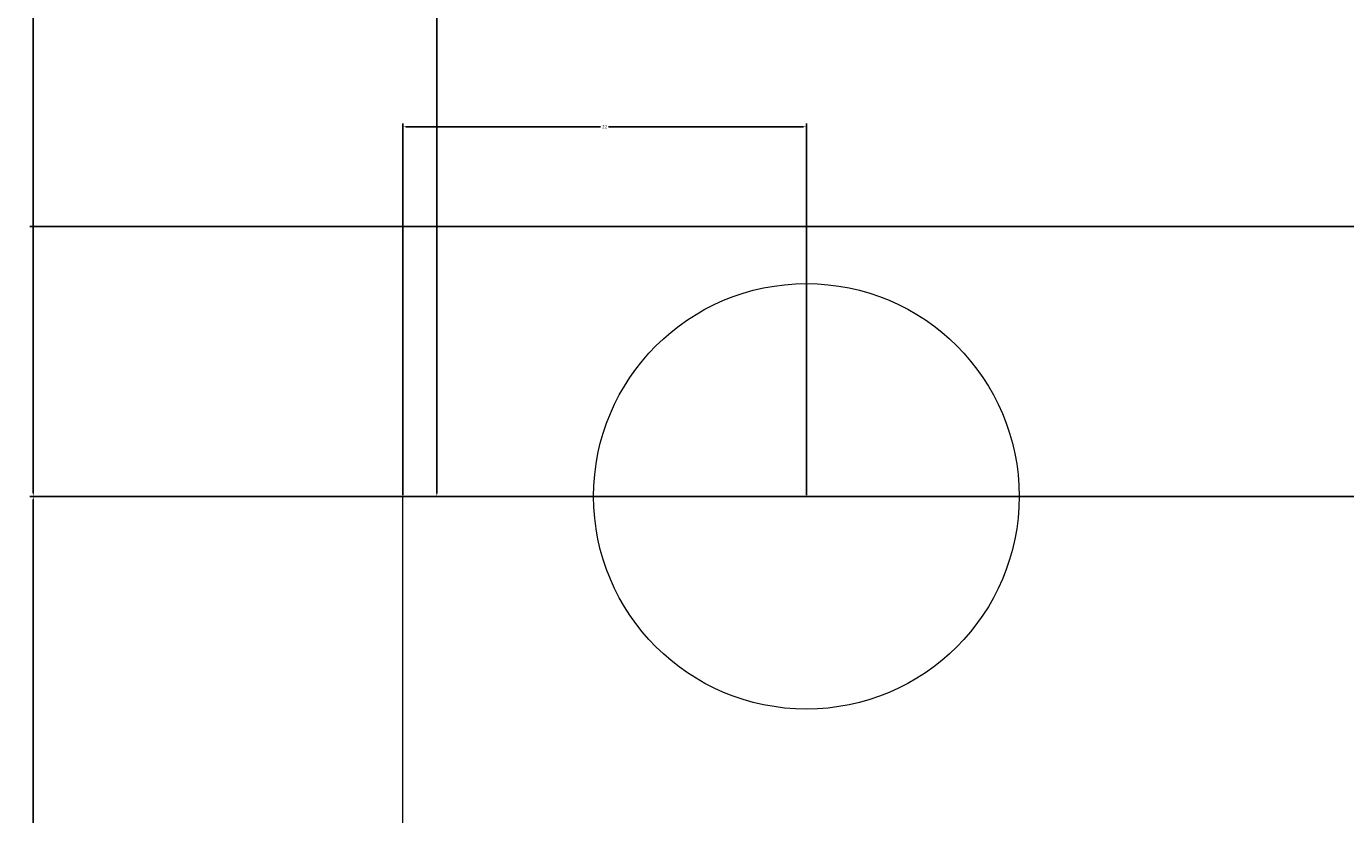
# Model space of a CAD drawing. Units: inches. Extents: x 1095 to 1408, y -20 to 240.
# Tile 2 of 8: x 1095 to 1167, y 23 to 66. Entities that reach past the tile are written whole.
import ezdxf

# ---------------------------------------------------------------- set-up
doc = ezdxf.new("R2010")
doc.units = ezdxf.units.IN
doc.header["$MEASUREMENT"] = 0
doc.layers.add('M-CONS', color=8, linetype='Continuous', lineweight=18)
doc.layers.add('M-DIMS', color=2, linetype='Continuous', lineweight=18)
doc.styles.get("Standard").update_dxf_attribs({"font": 'arial.ttf'})
doc.dimstyles.get("Standard").update_dxf_attribs({"dimtxt": 0.18, "dimasz": 0.18, "dimexe": 0.18, "dimexo": 0.0625, "dimgap": 0.09, "dimtad": 0, "dimtih": 1, "dimtoh": 1, "dimdec": 4, "dimzin": 0, "dimdsep": 46, "dimtxsty": 'Standard', "dimcen": 0.09, "dimadec": 0, "dimazin": 0, "dimtfac": 1, "dimtdec": 4, "dimtofl": 0, "dimtmove": 0, "dimatfit": 3, "dimfxl": 1, "dimtolj": 1, "dimtzin": 0, "dimarcsym": 0})

# ---------------------------------------------------------------- blocks, each defined once
blk = doc.blocks.new('*D3')
at = {"layer": 'Defpoints', "color": 0, "transparency": 16777216}
for p in [(1137.184, 60.15), (1115.184, 40), (1137.184, 40)]:
    blk.add_point(p, dxfattribs=at)
at = {"layer": 'M-DIMS', "color": 0, "lineweight": -2, "transparency": 16777216}
for p, q in [((1115.184, 40.062), (1115.184, 60.33)), ((1115.364, 60.15), (1125.964, 60.15)), ((1137.004, 60.15), (1126.403, 60.15)), ((1137.184, 40.062), (1137.184, 60.33))]:
    blk.add_line(p, q, dxfattribs=at)
at = {"layer": 'M-DIMS', "color": 0, "transparency": 16777216}
for points in [[(1115.364, 60.18), (1115.364, 60.12), (1115.184, 60.15)], [(1137.004, 60.18), (1137.004, 60.12), (1137.184, 60.15)]]:
    blk.add_solid(points, dxfattribs=at)
at = {"layer": 'M-DIMS', "color": 0, "transparency": 16777216, "insert": (1126.184, 60.15), "char_height": 0.18, "attachment_point": 5}
blk.add_mtext('\\A1;22', dxfattribs=at)
blk = doc.blocks.new('*D4')
at = {"layer": 'Defpoints', "color": 0, "transparency": 16777216}
for p in [(1095.034, 40), (1115.184, 40), (1115.184, 0)]:
    blk.add_point(p, dxfattribs=at)
at = {"layer": 'M-DIMS', "color": 0, "lineweight": -2, "transparency": 16777216}
for p, q in [((1115.121, 40), (1094.854, 40)), ((1095.034, 39.82), (1095.034, 20.182)), ((1095.034, 0.18), (1095.034, 19.818)), ((1115.121, 0), (1094.854, 0))]:
    blk.add_line(p, q, dxfattribs=at)
at = {"layer": 'M-DIMS', "color": 0, "transparency": 16777216}
for points in [[(1095.004, 39.82), (1095.064, 39.82), (1095.034, 40)], [(1095.004, 0.18), (1095.064, 0.18), (1095.034, 0)]]:
    blk.add_solid(points, dxfattribs=at)
at = {"layer": 'M-DIMS', "color": 0, "transparency": 16777216, "insert": (1095.034, 20), "char_height": 0.18, "attachment_point": 5}
blk.add_mtext('\\A1;40', dxfattribs=at)
blk = doc.blocks.new('*D6')
at = {"layer": 'Defpoints', "color": 0, "transparency": 16777216}
for p in [(1117.034, 208), (1137.184, 208), (1137.184, 40)]:
    blk.add_point(p, dxfattribs=at)
at = {"layer": 'M-DIMS', "color": 0, "lineweight": -2, "transparency": 16777216}
for p, q in [((1137.121, 208), (1116.854, 208)), ((1117.034, 207.82), (1117.034, 124.182)), ((1117.034, 40.18), (1117.034, 123.818)), ((1137.121, 40), (1116.854, 40))]:
    blk.add_line(p, q, dxfattribs=at)
at = {"layer": 'M-DIMS', "color": 0, "transparency": 16777216}
for points in [[(1117.004, 207.82), (1117.064, 207.82), (1117.034, 208)], [(1117.004, 40.18), (1117.064, 40.18), (1117.034, 40)]]:
    blk.add_solid(points, dxfattribs=at)
at = {"layer": 'M-DIMS', "color": 0, "transparency": 16777216, "insert": (1117.034, 124), "char_height": 0.18, "attachment_point": 5}
blk.add_mtext('\\A1;168', dxfattribs=at)
blk = doc.blocks.new('*D8')
at = {"layer": 'Defpoints', "color": 0, "transparency": 16777216}
for p in [(1095.034, 124), (1387.184, 124), (1365.184, 40)]:
    blk.add_point(p, dxfattribs=at)
at = {"layer": 'M-DIMS', "color": 0, "lineweight": -2, "transparency": 16777216}
for p, q in [((1387.121, 124), (1094.854, 124)), ((1095.034, 123.82), (1095.034, 82.182)), ((1095.034, 40.18), (1095.034, 81.818)), ((1365.121, 40), (1094.854, 40))]:
    blk.add_line(p, q, dxfattribs=at)
at = {"layer": 'M-DIMS', "color": 0, "transparency": 16777216}
for points in [[(1095.004, 123.82), (1095.064, 123.82), (1095.034, 124)], [(1095.004, 40.18), (1095.064, 40.18), (1095.034, 40)]]:
    blk.add_solid(points, dxfattribs=at)
at = {"layer": 'M-DIMS', "color": 0, "transparency": 16777216, "insert": (1095.034, 82), "char_height": 0.18, "attachment_point": 5}
blk.add_mtext('\\A1;84', dxfattribs=at)
blk = doc.blocks.new('*D10')
at = {"layer": 'Defpoints', "color": 0, "transparency": 16777216}
for p in [(1095.034, 193.282), (1211.184, 193.282), (1211.184, 54.718)]:
    blk.add_point(p, dxfattribs=at)
at = {"layer": 'M-DIMS', "color": 0, "lineweight": -2, "transparency": 16777216}
for p, q in [((1211.121, 193.282), (1094.854, 193.282)), ((1095.034, 193.102), (1095.034, 124.182)), ((1095.034, 54.898), (1095.034, 123.818)), ((1211.121, 54.718), (1094.854, 54.718))]:
    blk.add_line(p, q, dxfattribs=at)
at = {"layer": 'M-DIMS', "color": 0, "transparency": 16777216}
for points in [[(1095.004, 193.102), (1095.064, 193.102), (1095.034, 193.282)], [(1095.004, 54.898), (1095.064, 54.898), (1095.034, 54.718)]]:
    blk.add_solid(points, dxfattribs=at)
at = {"layer": 'M-DIMS', "color": 0, "transparency": 16777216, "insert": (1095.034, 124), "char_height": 0.18, "attachment_point": 5}
blk.add_mtext('\\A1;138.56', dxfattribs=at)

msp = doc.modelspace()

# ---------------------------------------------------------------- linework, layer by layer
at = {"layer": 'M-CONS'}
msp.add_line((1115.184, 0, 397.783), (1115.184, 40, 397.783), dxfattribs=at)
msp.add_circle((1137.184, 40, 397.783), 11.6, dxfattribs=at)

# ---------------------------------------------------------------- dimensions: what is measured, and where the dimension line sits
at = {"layer": 'M-DIMS'}
for base, p1, p2, override, picture, middle in [((1117.034, 208), (1137.184, 40), (1137.184, 208), {"dimdec": 0, "dimlfac": 1, "dimrnd": 0, "dimzin": 0, "dimdsep": 46, "dimlunit": 2}, '*D6', (1117.034, 124)), ((1095.034, 193.282), (1211.184, 54.718), (1211.184, 193.282), {"dimdec": 2, "dimlfac": 1, "dimrnd": 0, "dimzin": 0, "dimdsep": 46, "dimlunit": 2}, '*D10', (1095.034, 124)), ((1095.034, 124), (1365.184, 40), (1387.184, 124), {"dimdec": 0, "dimlfac": 1, "dimrnd": 0, "dimzin": 0, "dimdsep": 46, "dimlunit": 2}, '*D8', (1095.034, 82)), ((1095.034, 40), (1115.184, 0), (1115.184, 40), {"dimdec": 0, "dimlfac": 1, "dimrnd": 0, "dimzin": 0, "dimdsep": 46, "dimlunit": 2}, '*D4', (1095.034, 20))]:
    dim = msp.add_linear_dim(base=base, p1=p1, p2=p2, angle=90, dimstyle='Standard', override=override, dxfattribs=at)
    dim.commit()
    dim.dimension.update_dxf_attribs({"geometry": picture, "text_midpoint": middle})
dim = msp.add_linear_dim(base=(1137.184, 60.15), p1=(1115.184, 40), p2=(1137.184, 40), dimstyle='Standard', override={"dimdec": 0, "dimlfac": 1, "dimrnd": 0, "dimzin": 0, "dimdsep": 46, "dimlunit": 2}, dxfattribs=at)
dim.commit()
dim.dimension.update_dxf_attribs({"geometry": '*D3', "text_midpoint": (1126.184, 60.15)})

doc.saveas('drawing.dxf')
